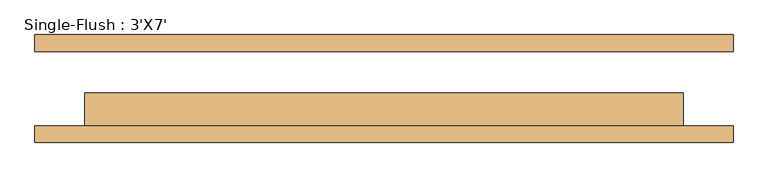
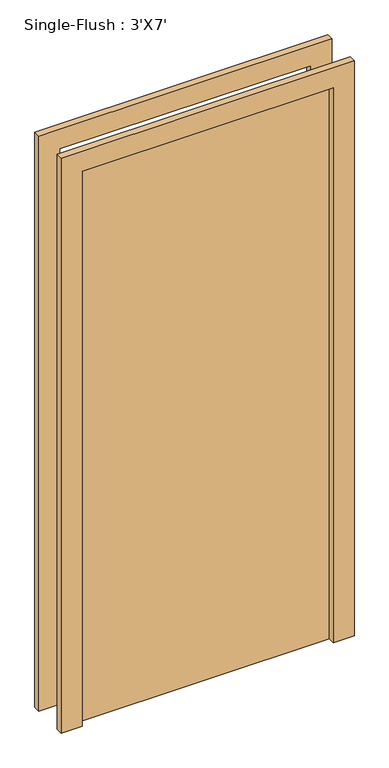
"""IFC4 building model written with IfcOpenShell, lengths in millimetres: door geometry, Single-Flush : 3'X7'."""

from ifc_helpers import new_model, si_unit, frame, origin, origin_with_axes, place, context, project, spatial, polyline, outline, extrude, source, transform, mapped, element, save


def single_flush_3_x7_305aa2a5(model_context):
    return source(origin(), model_context, "Body", "SweptSolid", [
        extrude(outline(polyline([(2209.8, -533.4), (0.0, -533.4), (0.0, -457.2), (2133.6, -457.2), (2133.6, 457.2), (0.0, 457.2), (0.0, 533.4), (2209.8, 533.4), (2209.8, -533.4)])), frame((0.0, -82.55, 0.0), z_axis=(0.0, 1.0, 0.0), x_axis=(0.0, 0.0, 1.0)), (0.0, 0.0, 1.0), 25.4),
        extrude(outline(polyline([(2209.8, 533.4), (2209.8, -533.4), (0.0, -533.4), (0.0, -457.2), (2133.6, -457.2), (2133.6, 457.2), (0.0, 457.2), (0.0, 533.4), (2209.8, 533.4)])), frame((0.0, 57.15, 0.0), z_axis=(0.0, 1.0, 0.0), x_axis=(0.0, 0.0, 1.0)), (0.0, 0.0, 1.0), 25.4),
        extrude(outline(polyline([(457.2, -6.35), (457.2, -57.15), (-457.2, -57.15), (-457.2, -6.35), (457.2, -6.35)])), origin_with_axes(), (0.0, 0.0, 1.0), 2133.6),
    ])


if __name__ == "__main__":
    model = new_model("IFC4")
    model_context = context("Model", 3, world=origin())
    ifc_project = project(units=[si_unit("LENGTHUNIT", "METRE", prefix="MILLI")], contexts=[model_context])
    site = spatial("IfcSite", under=ifc_project)
    building = spatial("IfcBuilding", under=site)
    placement = place(None, origin())
    single_flush_3_x7_shape = single_flush_3_x7_305aa2a5(model_context)
    element("IfcDoor", 1, ObjectType="Single-Flush : 3'X7'", at=placement, inside=building, context=model_context, shape_type="MappedRepresentation", body=[
        mapped(single_flush_3_x7_shape, transform((0.0, 0.0, 0.0), x_axis=(1.0, 0.0, 0.0), y_axis=(0.0, 1.0, 0.0), z_axis=(0.0, 0.0, 1.0))),
    ])
    save(model, "model.ifc")

# Revit data of these elements
# Type "Single-Flush : 3'X7'"
#   Type Mark = "8"
#   Construction Type Id = "MDOOR"
#   Assembly Code = "C1020"
#   Analytic Construction = "Metal"
#   Thickness = 0' - 2"
#   Heat Transfer Coefficient (U) = 0.651978 BTU/(h·ft²·°F)
#   Height = 7' - 0"
#   Trim Projection Ext = 0' - 1"
#   Trim Projection Int = 0' - 1"
#   Trim Width = 0' - 3"
#   Width = 3' - 0"
#   Define Thermal Properties by = 1
#   Door Material = Door - Panel
#   Frame Material = Door - Frame
#   Visual Light Transmittance = 0
#   Solar Heat Gain Coefficient = 0
#   Function = (empty or 0)
#   Wall Closure = (empty or 0)
# Element 1 (IfcDoor, "Single-Flush : 3'X7'")
#   Materials on its faces: "Door - Frame", "Door - Panel"
# Materials
#   "Door - Panel": class "Wood", colour RGB 210 159 95, transparency 0, Cost = 0
#   "Door - Frame": colour RGB 118 70 51, transparency 0, Cost = 0
